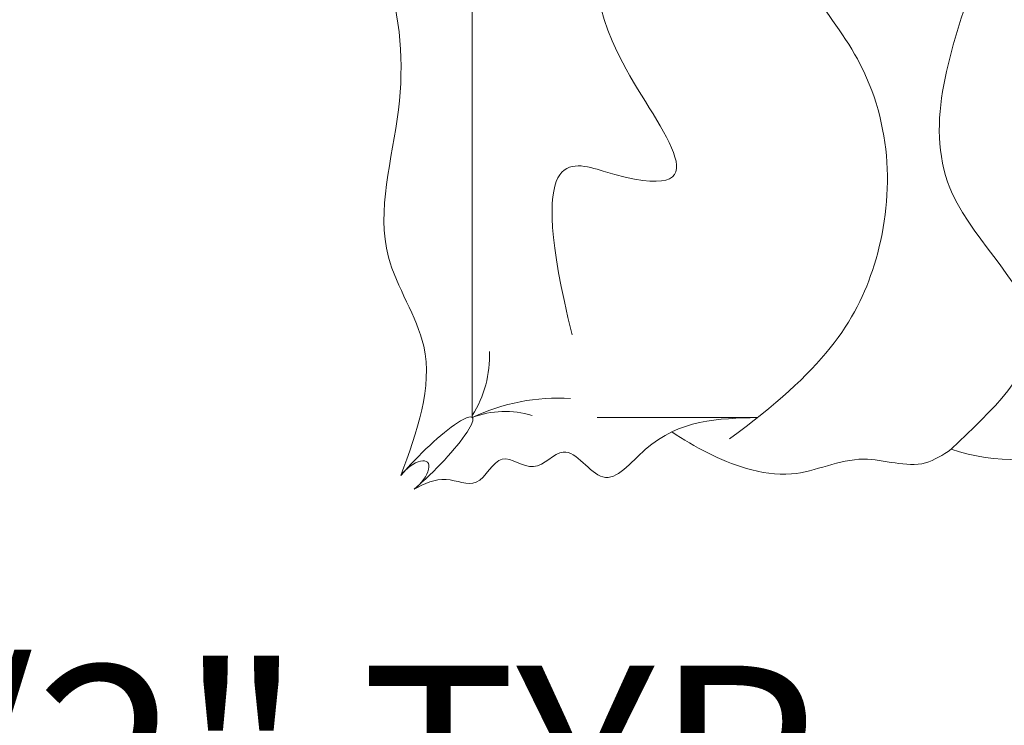
# Model space of a CAD drawing. Units: inches. Extents: x 2083 to 3317, y 1141 to 2115.
# Tile 120 of 256: x 3006 to 3068, y 1283 to 1327. Entities that reach past the tile are written whole.
import ezdxf

# ---------------------------------------------------------------- set-up
doc = ezdxf.new("R2010")
doc.units = ezdxf.units.IN
for name, color, linetype, lineweight in [('A-ANNO-DIMS', 2, 'Continuous', 18), ('A-FURN', 8, 'Continuous', 18), ('www.cadblocksfree.com', 7, 'Continuous', 9)]:
    doc.layers.add(name, color=color, linetype=linetype, lineweight=lineweight)
doc.layers.add('A-WALL-PATT', color=251, linetype='Continuous', lineweight=13, true_color=0x636466)
doc.styles.get("Standard").update_dxf_attribs({"font": 'arial.ttf'})
doc.dimstyles.new('ISO-25', dxfattribs={"dimtxt": 12, "dimasz": 12, "dimexe": 1.25, "dimexo": 0.625, "dimtad": 1, "dimlunit": 3, "dimtxsty": 'Standard', "dimcen": 2.5, "dimadec": 0, "dimazin": 0, "dimtfac": 1, "dimtmove": 0, "dimatfit": 3, "dimfxl": 1, "dimarcsym": 0})

# ---------------------------------------------------------------- blocks, each defined once
blk = doc.blocks.new('bed')
at = {"layer": 'www.cadblocksfree.com', "ltscale": 0.2}
for p, q in [((3426.379, 1399.908), (3426.379, 1410.814)), ((3363.387, 1391.414), (3426.379, 1391.414))]:
    blk.add_line(p, q, dxfattribs=at)
for centre, radius, start, end in [((3416.575, 1428.082), 12.646, 341.02679, 23.77822), ((3438.819, 1397.314), 13.768, 176.75247, 205.37301), ((3432.135, 1393.639), 6.173, 162.64747, 201.1361), ((3422.111, 1384.801), 7.798, 58.00129, 91.65506)]:
    blk.add_arc(centre, radius, start, end, dxfattribs=at)
for centre, major_axis, ratio, start_param, end_param in [((3429.422, 1388.371), (-3.043, 3.043), 0.168252, 4.250342, 8.316029), ((3430.477, 1387.316), (-1.055, 1.055), 0.453532, 4.422107, 8.144264)]:
    blk.add_ellipse(centre, major_axis=major_axis, ratio=ratio, start_param=start_param, end_param=end_param, dxfattribs=at)
for points, knots in [([(3365.512, 1424.213), (3370.519, 1427.004), (3381.149, 1429.825), (3396.214, 1425.866), (3410.541, 1420.654), (3420.273, 1432.695), (3425.882, 1426.771), (3428.534, 1423.97)], [0.099185, 0.099185, 0.099185, 0.099185, 0.523647, 0.927087, 1.289918, 1.564439, 1.810555, 1.810555, 1.810555, 1.810555]), ([(3428.534, 1423.97), (3428.914, 1423.397), (3430.098, 1421.613), (3428.491, 1417.656), (3430.593, 1413.794), (3429.801, 1409.122), (3428.396, 1406.564), (3427.355, 1404.971)], [0, 0, 0, 0, 0.050513, 0.157399, 0.2842023, 0.3628173, 0.5066917, 0.5066917, 0.5066917, 0.5066917]), ([(3362.057, 1409.866), (3363.638, 1413.65), (3372.978, 1421.337), (3389.682, 1406.045), (3402.396, 1419.984), (3416.037, 1420.167), (3423.233, 1415.231), (3427.827, 1408.899)], [0.029901, 0.029901, 0.029901, 0.029901, 0.276967, 0.797115, 1.093669, 1.464666, 1.788489, 1.788489, 1.788489, 1.788489]), ([(3431.237, 1387.473), (3430.882, 1388.172), (3430.205, 1389.505), (3431.478, 1391.985), (3428.294, 1393.194), (3430.501, 1395.689), (3427.558, 1397.866), (3431.841, 1400.386), (3426.535, 1404.33), (3426.443, 1408.152), (3426.379, 1410.814)], [0, 0, 0, 0, 2.267059, 4.324559, 6.685584, 8.878641, 11.121502, 14.300359, 17.755284, 25.682856, 25.682856, 25.682856, 25.682856]), ([(3368.632, 1397.839), (3375.978, 1400.489), (3385.349, 1402.757), (3397.531, 1395.273), (3413.593, 1410.377), (3407.806, 1395.019), (3420.759, 1398.2)], [0.029901, 0.029901, 0.029901, 0.029901, 0.276967, 0.797115, 1.093669, 1.16836, 1.16836, 1.16836, 1.16836]), ([(3430.32, 1386.556), (3427.327, 1387.653), (3422.148, 1389.55), (3414.529, 1384.137), (3405.607, 1387.046), (3396.29, 1386.314), (3386.838, 1381.282), (3377.742, 1390.272), (3370.778, 1384.799), (3364.626, 1383.966), (3363.275, 1388.265), (3360.778, 1387.151), (3359.446, 1386.556)], [0, 0, 0, 0, 8.93042, 15.449194, 25.485629, 34.878505, 43.598887, 54.554403, 64.16647, 67.461673, 70.610457, 74.213583, 74.213583, 74.213583, 74.213583])]:
    blk.add_open_spline(points, degree=3, knots=knots, dxfattribs=at)
blk = doc.blocks.new('*D26')
at = {"layer": 'A-ANNO-DIMS', "color": 0, "lineweight": -2, "transparency": 16777216}
for p, q in [((3088.986, 1274.915), (3088.986, 1270.952)), ((3111.24, 1274.915), (3111.24, 1270.952)), ((3076.986, 1272.202), (2840.262, 1272.202)), ((3111.24, 1272.202), (3088.986, 1272.202)), ((3123.24, 1272.202), (3135.24, 1272.202))]:
    blk.add_line(p, q, dxfattribs=at)
at = {"layer": 'A-ANNO-DIMS', "color": 0, "transparency": 16777216}
for points in [[(3076.986, 1274.202), (3076.986, 1270.202), (3088.986, 1272.202)], [(3123.24, 1274.202), (3123.24, 1270.202), (3111.24, 1272.202)]]:
    blk.add_solid(points, dxfattribs=at)
at = {"layer": 'Defpoints', "color": 0, "transparency": 16777216}
for p in [(3088.986, 1275.54), (3111.24, 1275.54), (3088.986, 1272.202)]:
    blk.add_point(p, dxfattribs=at)
at = {"layer": 'A-ANNO-DIMS', "color": 0, "transparency": 16777216, "insert": (2952.624, 1279.032), "char_height": 12, "attachment_point": 5}
blk.add_mtext('NIGHTSTAND 1\'-10 1/2" TYP.', dxfattribs=at)

msp = doc.modelspace()

# ---------------------------------------------------------------- hatches: boundary and pattern name
at = {"layer": 'A-WALL-PATT'}
h = msp.add_hatch(color=256, dxfattribs=at)
h.dxf.hatch_style = 1
h.paths.add_polyline_path([(3126.96, 2020.761), (2748.96, 2020.761), (2604.96, 2020.761), (2226.96, 2020.761), (2226.96, 1702.761), (2466.96, 1702.761), (2466.96, 1582.761), (2418.96, 1582.761), (2418.96, 1477.761), (2226.96, 1477.761), (2226.96, 1263.261), (2544.96, 1263.261), (2544.96, 1411.761), (2604.96, 1411.761), (2685.96, 1411.761), (2685.96, 1420.761), (2604.96, 1420.761), (2604.96, 1573.761), (2604.96, 1702.761), (2604.96, 2011.761), (2748.96, 2011.761), (2748.96, 1702.761), (2862.96, 1702.761), (2862.96, 1621.761), (2871.96, 1621.761), (2871.96, 1702.761), (2883.96, 1702.761), (2883.96, 1706.939, -0.026459), (2883.96, 1711.761), (2757.96, 1711.761), (2757.96, 1807.761), (2787.96, 1807.761), (2787.96, 1812.261), (2757.96, 1812.261), (2757.96, 2011.761), (2877.96, 2011.761), (2877.96, 1812.261), (2847.96, 1812.261), (2847.96, 1807.761), (2889.836, 1807.761), (2889.836, 1812.261), (2882.46, 1812.261), (2882.46, 2011.761), (3117.96, 2011.761), (3117.96, 1812.261), (2937.836, 1812.261), (2937.836, 1807.761), (2995.71, 1807.761), (2995.71, 1796.118), (3000.21, 1796.118), (3000.21, 1807.761), (3117.96, 1807.761), (3117.96, 1711.761), (3000.21, 1711.761), (3000.21, 1760.118), (2998.573, 1760.118, -0.020711), (2995.71, 1760.118), (2995.71, 1711.761), (2931.96, 1711.761), (2931.96, 1702.761), (3126.96, 1702.761)])
h.paths.add_polyline_path([(2471.46, 2011.761), (2471.46, 1810.011), (2462.717, 1810.011), (2462.717, 1805.511), (2505.96, 1805.511), (2505.96, 1810.011), (2475.96, 1810.011), (2475.96, 2011.761), (2595.96, 2011.761), (2595.96, 1810.011), (2565.96, 1810.011), (2565.96, 1805.511), (2595.96, 1805.511), (2595.96, 1711.761), (2235.96, 1711.761), (2235.96, 1805.511), (2353.71, 1805.511), (2353.71, 1796.054), (2358.21, 1796.054), (2358.21, 1805.511), (2414.717, 1805.511), (2414.717, 1810.011), (2235.96, 1810.011), (2235.96, 2011.761)], flags=16)
h.paths.add_polyline_path([(2270.205, 1994.61), (2270.205, 1970.61), (2246.205, 1970.61), (2246.205, 1994.61)], flags=0)
edge = h.paths.add_edge_path(flags=0)
edge.add_ellipse((2332.027, 1899.798), major_axis=(-3.043, 3.043), ratio=0.168252, start_angle=-161.33217, end_angle=-156.30711, ccw=False)
edge.add_ellipse((2333.082, 1898.744), major_axis=(-1.055, 1.055), ratio=0.453532, start_angle=-123.37102, end_angle=-94.15911)
edge = h.paths.add_edge_path(flags=0)
edge.add_ellipse((2332.027, 1968.876), major_axis=(3.043, 3.043), ratio=0.168252, start_angle=18.66783, end_angle=23.69289)
edge.add_spline(control_points=[(2332.926, 1970.691), (2332.227, 1970.336), (2330.894, 1969.659), (2328.413, 1970.932), (2327.204, 1967.749), (2324.71, 1969.956), (2322.533, 1967.012), (2320.013, 1971.296), (2317.68, 1968.158), (2316.041, 1967.102), (2315.427, 1966.81)], knot_values=[0, 0, 0, 0, 2.267059, 4.324559, 6.685584, 8.878641, 11.121502, 14.300359, 17.755284, 19.732645, 19.732645, 19.732645, 19.732645], degree=3, periodic=0)
edge.add_ellipse((2332.027, 1968.876), major_axis=(3.043, 3.043), ratio=0.168252, start_angle=18.66783, end_angle=23.69289, ccw=False)
edge.add_ellipse((2333.082, 1969.931), major_axis=(1.055, 1.055), ratio=0.453532, start_angle=56.62898, end_angle=85.84089, ccw=False)
edge = h.paths.add_edge_path(flags=0)
edge.add_spline(control_points=[(2296.428, 1967.988), (2293.628, 1965.336), (2287.704, 1959.727), (2299.744, 1949.996), (2294.533, 1935.669), (2290.573, 1920.604), (2293.394, 1909.974), (2296.185, 1904.967)], knot_values=[0.099185, 0.099185, 0.099185, 0.099185, 0.345301, 0.619822, 0.982653, 1.386093, 1.810555, 1.810555, 1.810555, 1.810555], degree=3, periodic=0)
edge.add_spline(control_points=[(2296.185, 1904.967), (2297.384, 1902.619), (2298.001, 1901.949), (2298.553, 1901.468)], knot_values=[0.006246, 0.006246, 0.006246, 0.006246, 0.055476, 0.055476, 0.055476, 0.055476], degree=3, periodic=0)
edge.add_spline(control_points=[(2298.553, 1901.468), (2297.259, 1900.923), (2295.225, 1900.232), (2293.06, 1900.614), (2292.101, 1900.788), (2292.09, 1900.791)], knot_values=[0.312835, 0.312835, 0.312835, 0.312835, 0.40178, 0.474987, 0.475903, 0.475903, 0.475903, 0.475903], degree=3, periodic=0)
edge.add_arc((2292.794, 1904.664), 3.937, 215.4209, 259.69818, ccw=False)
edge.add_spline(control_points=[(2289.585, 1902.382), (2289.477, 1902.535), (2289.368, 1902.688), (2289.261, 1902.841)], knot_values=[0.102872, 0.102872, 0.102872, 0.102872, 0.116896, 0.116896, 0.116896, 0.116896], degree=3, periodic=0)
edge.add_spline(control_points=[(2289.261, 1902.841), (2288.687, 1902.55), (2287.64, 1902.02), (2285.881, 1901.874), (2283.853, 1901.504), (2281.72, 1899.711), (2278.467, 1899.493), (2276.157, 1901.883), (2272.259, 1899.804), (2267.778, 1901.843), (2262.244, 1900.184), (2257.415, 1901.782), (2254.318, 1900.726), (2253.178, 1900.337)], knot_values=[0, 0, 0, 0, 1.907977, 3.477176, 5.261074, 7.972851, 11.680248, 13.717921, 16.939592, 22.789562, 27.502503, 33.595215, 37.145618, 37.145618, 37.145618, 37.145618], degree=3, periodic=0)
edge.add_line((2253.178, 1900.337), (2250.244, 1902.841))
edge.add_line((2250.244, 1902.841), (2250.244, 1965.833))
edge.add_line((2250.244, 1965.833), (2253.178, 1968.337))
edge.add_spline(control_points=[(2253.178, 1968.337), (2254.318, 1967.948), (2257.415, 1966.892), (2262.244, 1968.49), (2267.778, 1966.831), (2271.527, 1968.537), (2273.876, 1967.828), (2274.207, 1967.728)], knot_values=[0, 0, 0, 0, 0.09018, 0.244935, 0.364644, 0.513233, 0.537855, 0.537855, 0.537855, 0.537855], degree=3, periodic=0)
edge.add_arc((2274.353, 1963.793), 3.937, 72.05113, 92.12795, ccw=False)
edge.add_arc((2281.297, 1985.23), 18.596, 252.05113, 288.56572)
edge.add_arc((2292.317, 1956.029), 12.646, 71.02679, 113.77822, ccw=False)
edge = h.paths.add_edge_path(flags=0)
edge.add_spline(control_points=[(2274.899, 1951.856), (2275.066, 1951.617), (2275.233, 1951.377), (2275.398, 1951.136)], knot_values=[1.409916, 1.409916, 1.409916, 1.409916, 1.43159, 1.43159, 1.43159, 1.43159], degree=3, periodic=0)
edge.add_spline(control_points=[(2275.398, 1951.136), (2275.792, 1950.562), (2276.179, 1949.984), (2276.546, 1949.397)], knot_values=[1.358238, 1.358238, 1.358238, 1.358238, 1.409916, 1.409916, 1.409916, 1.409916], degree=3, periodic=0)
edge.add_line((2276.546, 1949.397), (2277.437, 1947.862))
edge.add_spline(control_points=[(2277.437, 1947.862), (2276.304, 1945.673), (2274.64, 1942.427), (2274.632, 1938.094), (2272.799, 1930.852), (2274.356, 1943.897), (2275.948, 1947.923), (2276.546, 1949.397)], knot_values=[0.005632, 0.005632, 0.005632, 0.005632, 0.186014, 0.266002, 0.357087, 0.59639, 0.739732, 0.739732, 0.739732, 0.739732], degree=3, periodic=0)
edge.add_spline(control_points=[(2276.546, 1949.397), (2276.179, 1949.984), (2275.792, 1950.562), (2275.398, 1951.136)], knot_values=[1.358238, 1.358238, 1.358238, 1.358238, 1.409916, 1.409916, 1.409916, 1.409916], degree=3, periodic=0)
edge.add_spline(control_points=[(2275.398, 1951.136), (2274.943, 1950.08), (2274.208, 1948.025), (2273.935, 1944.851), (2272.469, 1937.627), (2273.466, 1945.696), (2274.701, 1951.059), (2274.899, 1951.856)], knot_values=[0.104364, 0.104364, 0.104364, 0.104364, 0.189636, 0.269624, 0.36071, 0.600013, 0.644622, 0.644622, 0.644622, 0.644622], degree=3, periodic=0)
h.paths.add_polyline_path([(2269.168, 1963.128, -0.357527), (2268.171, 1960.976, -0.092561), (2268.171, 1939.436, -0.357527), (2269.168, 1937.285, -0.357527), (2267.016, 1938.282, -0.164785), (2254.686, 1938.282, -0.357527), (2252.534, 1937.285, -0.357527), (2253.531, 1939.436, -0.092561), (2253.531, 1960.976, -0.357527), (2252.534, 1963.128, -0.357527), (2254.686, 1962.131, -0.164785), (2267.016, 1962.131, -0.357527)], flags=0)
h.paths.add_polyline_path([(2248.874, 1967.802), (2248.874, 1957.028), (2249.458, 1957.028), (2249.458, 1911.647), (2248.874, 1911.647), (2248.874, 1900.873), (2246.512, 1900.873, 0.197327), (2244.15, 1902.457), (2244.15, 1966.218, 0.197327), (2246.512, 1967.802)], flags=0)
h.paths.add_polyline_path([(2269.168, 1931.389, -0.357527), (2268.171, 1929.238, -0.092561), (2268.171, 1907.698, -0.357527), (2269.168, 1905.547, -0.357527), (2267.016, 1906.544, -0.164785), (2254.686, 1906.544, -0.357527), (2252.534, 1905.547, -0.357527), (2253.531, 1907.698, -0.092561), (2253.531, 1929.238, -0.357527), (2252.534, 1931.389, -0.357527), (2254.686, 1930.392, -0.164785), (2267.016, 1930.392, -0.357527)], flags=0)
edge = h.paths.add_edge_path(flags=0)
edge.add_spline(control_points=[(2276.197, 1906.724), (2276.168, 1909.029), (2276.114, 1913.372), (2270.598, 1924.925), (2273.905, 1919.013), (2275.922, 1916.262), (2275.475, 1912.402), (2277.258, 1910.381), (2276.696, 1908.225), (2276.646, 1906.813), (2276.618, 1906.008)], knot_values=[0, 0, 0, 0, 8.61026, 16.221274, 18.843057, 23.804898, 27.440828, 29.356102, 31.203478, 33.650687, 33.650687, 33.650687, 33.650687], degree=3, periodic=0)
edge.add_spline(control_points=[(2276.618, 1906.008), (2276.623, 1905.624), (2276.498, 1904.629), (2275.442, 1903.855), (2274.937, 1903.08), (2274.859, 1902.841)], knot_values=[0.156488, 0.156488, 0.156488, 0.156488, 0.184398, 0.231376, 0.250598, 0.250598, 0.250598, 0.250598], degree=3, periodic=0)
edge.add_line((2274.859, 1902.841), (2276.506, 1902.841))
edge.add_spline(control_points=[(2276.506, 1902.841), (2276.788, 1903.085), (2277.665, 1904.125), (2278.25, 1904.341), (2277.654, 1908.527), (2278.156, 1906.228), (2278.1, 1905.286), (2278.847, 1904.069), (2277.857, 1903.415), (2277.874, 1902.991), (2277.904, 1902.841)], knot_values=[0.059574, 0.059574, 0.059574, 0.059574, 0.080753, 0.103741, 0.16972, 0.176036, 0.207137, 0.240474, 0.262341, 0.27366, 0.27366, 0.27366, 0.27366], degree=3, periodic=0)
edge.add_line((2277.904, 1902.841), (2280.03, 1902.841))
edge.add_spline(control_points=[(2280.03, 1902.841), (2279.888, 1903.088), (2279.499, 1903.982), (2280.152, 1905.939), (2278.104, 1909.658), (2279.762, 1907.185), (2280.328, 1904.875), (2280.485, 1903.49), (2281.463, 1903.249), (2281.758, 1902.936), (2281.834, 1902.841)], knot_values=[0.013856, 0.013856, 0.013856, 0.013856, 0.034874, 0.088867, 0.107879, 0.126738, 0.158714, 0.193757, 0.217487, 0.226722, 0.226722, 0.226722, 0.226722], degree=3, periodic=0)
edge.add_spline(control_points=[(2281.834, 1902.841), (2281.788, 1902.827), (2281.647, 1902.783), (2281.396, 1902.859), (2281.088, 1902.985), (2280.721, 1903.061), (2280.333, 1903.026), (2280.125, 1902.899), (2280.03, 1902.841)], knot_values=[0, 0, 0, 0, 0.14413, 0.435517, 0.749276, 1.153046, 1.548371, 1.878348, 1.878348, 1.878348, 1.878348], degree=3, periodic=0)
edge.add_line((2280.03, 1902.841), (2277.904, 1902.841))
edge.add_spline(control_points=[(2277.904, 1902.841), (2277.893, 1902.796), (2277.865, 1902.68), (2277.607, 1902.687), (2277.274, 1902.801), (2276.838, 1902.62), (2276.584, 1902.789), (2276.506, 1902.841)], knot_values=[0, 0, 0, 0, 0.127189, 0.326199, 0.628009, 1.24357, 1.515331, 1.515331, 1.515331, 1.515331], degree=3, periodic=0)
edge.add_line((2276.506, 1902.841), (2274.859, 1902.841))
edge.add_spline(control_points=[(2274.859, 1902.841), (2274.814, 1902.899), (2274.725, 1903.013), (2274.493, 1903.119), (2274.244, 1902.961), (2273.937, 1903.185), (2273.614, 1902.983), (2273.408, 1902.883), (2273.322, 1902.841)], knot_values=[0, 0, 0, 0, 0.21843, 0.436957, 0.687977, 0.990379, 1.398396, 1.69185, 1.69185, 1.69185, 1.69185], degree=3, periodic=0)
edge.add_spline(control_points=[(2273.322, 1902.841), (2273.617, 1903.446), (2274.274, 1904.538), (2276.027, 1904.574), (2276.207, 1906.584), (2276.197, 1906.724)], knot_values=[0.012227, 0.012227, 0.012227, 0.012227, 0.059472, 0.106218, 0.134458, 0.134458, 0.134458, 0.134458], degree=3, periodic=0)
h.paths.add_polyline_path([(2270.776, 1897.79), (2270.776, 1873.79), (2246.776, 1873.79), (2246.776, 1897.79)], flags=0)
h.paths.add_polyline_path([(2353.71, 1760.005), (2353.71, 1760.054), (2358.21, 1760.054, -0.033729)], flags=0)
h.paths.add_polyline_path([(2321.819, 1737.529), (2341.995, 1737.529, -0.414214), (2343.203, 1736.321), (2343.203, 1721.021, -0.414214), (2341.995, 1719.813), (2321.819, 1719.813, -0.414214), (2320.611, 1721.021), (2320.611, 1736.321, -0.414214)], flags=0)
h.paths.add_polyline_path([(2324.235, 1736.321), (2339.579, 1736.321, -0.414214), (2341.995, 1733.905), (2341.995, 1725.45, -0.414214), (2339.579, 1723.034), (2333.681, 1723.034), (2333.845, 1722.045, -0.870646), (2335.425, 1721.826, -0.767327), (2333.923, 1721.423), (2331.291, 1721.423, -0.767327), (2329.788, 1721.826, -0.870646), (2331.368, 1722.045), (2331.533, 1723.034), (2324.235, 1723.034, -0.414214), (2321.819, 1725.45), (2321.819, 1733.905, -0.414214)], flags=0)
h.paths.add_polyline_path([(2570.484, 1928.615), (2589.684, 1928.615), (2590.169, 1928.615), (2590.169, 1904.993), (2570.484, 1904.993)], flags=0)
h.paths.add_polyline_path([(2574.447, 1927.264, -1), (2572.829, 1927.264, -1)], flags=0)
h.paths.add_polyline_path([(2573.09, 1926.941), (2573.925, 1927.776), (2574.148, 1927.553), (2573.313, 1926.718)], flags=0)
h.paths.add_polyline_path([(2578.779, 1919.73, -1), (2571.592, 1919.73, -1)], flags=0)
h.paths.add_polyline_path([(2578.385, 1919.73, -1), (2571.985, 1919.73, -1)], flags=0)
h.paths.add_polyline_path([(2331.596, 1729.476, -1), (2333.618, 1729.476, -1)], flags=0)
h.paths.add_polyline_path([(2578.034, 1927.264, -1), (2576.416, 1927.264, -1)], flags=0)
h.paths.add_polyline_path([(2576.689, 1927.531), (2576.912, 1927.754), (2577.747, 1926.919), (2577.524, 1926.696)], flags=0)
h.paths.add_polyline_path([(2578.139, 1909.86, -1), (2572.232, 1909.86, -1)], flags=0)
h.paths.add_polyline_path([(2577.745, 1909.86, -1), (2572.625, 1909.86, -1)], flags=0)
h.paths.add_polyline_path([(2583.798, 1927.264, -1), (2582.179, 1927.264, -1)], flags=0)
h.paths.add_polyline_path([(2582.719, 1927.754), (2583.554, 1926.919), (2583.331, 1926.696), (2582.496, 1927.531)], flags=0)
h.paths.add_polyline_path([(2582.496, 1927.531), (2582.719, 1927.754), (2583.554, 1926.919), (2583.331, 1926.696)], flags=0)
h.paths.add_polyline_path([(2587.739, 1920.53, -1), (2581.832, 1920.53, -1)], flags=0)
h.paths.add_polyline_path([(2587.345, 1920.53, -1), (2582.225, 1920.53, -1)], flags=0)
h.paths.add_polyline_path([(2587.385, 1927.264, -1), (2585.766, 1927.264, -1)], flags=0)
h.paths.add_polyline_path([(2586.082, 1926.98), (2586.917, 1927.815), (2587.14, 1927.593), (2586.305, 1926.758)], flags=0)
h.paths.add_polyline_path([(2588.379, 1910.66, -1), (2581.192, 1910.66, -1)], flags=0)
h.paths.add_polyline_path([(2587.985, 1910.66, -1), (2581.585, 1910.66, -1)], flags=0)
h.paths.add_polyline_path([(2417.168, 1729.478), (2437.344, 1729.478, -0.414214), (2438.552, 1728.27), (2438.552, 1712.969, -0.414214), (2437.344, 1711.761), (2417.168, 1711.761, -0.414214), (2415.96, 1712.969), (2415.96, 1728.27, -0.414214)], flags=0)
h.paths.add_polyline_path([(2419.584, 1728.27), (2434.928, 1728.27, -0.414214), (2437.344, 1725.854), (2437.344, 1717.398, -0.414214), (2434.928, 1714.983), (2429.029, 1714.983), (2429.194, 1713.994, -0.870646), (2430.774, 1713.775, -0.767327), (2429.271, 1713.372), (2426.64, 1713.372, -0.767327), (2425.137, 1713.775, -0.870646), (2426.717, 1713.994), (2426.882, 1714.983), (2419.584, 1714.983, -0.414214), (2417.168, 1717.398), (2417.168, 1725.854, -0.414214)], flags=0)
h.paths.add_polyline_path([(2419.584, 1728.27), (2434.928, 1728.27, -0.414214), (2437.344, 1725.854), (2437.344, 1717.398, -0.414214), (2434.928, 1714.983), (2429.029, 1714.983), (2428.358, 1719.009), (2427.553, 1719.009), (2426.882, 1714.983), (2419.584, 1714.983, -0.414214), (2417.168, 1717.398), (2417.168, 1725.854, -0.414214)], flags=0)
h.paths.add_polyline_path([(2426.944, 1721.425, -1), (2428.967, 1721.425, -1)], flags=0)
h.paths.add_polyline_path([(2475.96, 1702.761), (2595.96, 1702.761), (2595.96, 1582.761), (2475.96, 1582.761)], flags=16)
h.paths.add_polyline_path([(2427.96, 1573.761), (2595.96, 1573.761), (2595.96, 1468.761), (2595.96, 1420.761), (2384.46, 1420.761), (2384.46, 1468.761), (2427.96, 1468.761)], flags=16)
h.paths.add_polyline_path([(2379.96, 1468.761), (2379.96, 1420.761), (2235.96, 1420.761), (2235.96, 1468.761)], flags=16)
h.paths.add_polyline_path([(2317.816, 1466.696), (2337.992, 1466.696, -0.414214), (2339.2, 1465.488), (2339.2, 1450.187, -0.414214), (2337.992, 1448.979), (2317.816, 1448.979, -0.414214), (2316.608, 1450.187), (2316.608, 1465.488, -0.414214)], flags=0)
h.paths.add_polyline_path([(2320.232, 1465.488), (2335.576, 1465.488, -0.414214), (2337.992, 1463.072), (2337.992, 1454.616, -0.414214), (2335.576, 1452.2), (2329.677, 1452.2), (2329.842, 1451.212, -0.870646), (2331.422, 1450.992, -0.767327), (2329.92, 1450.59), (2327.288, 1450.59, -0.767327), (2325.785, 1450.992, -0.870646), (2327.365, 1451.212), (2327.53, 1452.2), (2320.232, 1452.2, -0.414214), (2317.816, 1454.616), (2317.816, 1463.072, -0.414214)], flags=0)
h.paths.add_polyline_path([(2320.232, 1465.488), (2335.576, 1465.488, -0.414214), (2337.992, 1463.072), (2337.992, 1454.616, -0.414214), (2335.576, 1452.2), (2329.677, 1452.2), (2329.006, 1456.227), (2328.201, 1456.227), (2327.53, 1452.2), (2320.232, 1452.2, -0.414214), (2317.816, 1454.616), (2317.816, 1463.072, -0.414214)], flags=0)
h.paths.add_polyline_path([(2327.593, 1458.643, -1), (2329.615, 1458.643, -1)], flags=0)
h.paths.add_polyline_path([(2244.412, 1433.34), (2241.921, 1433.34, -0.414214), (2240.018, 1435.244), (2240.018, 1440.953, -0.414211), (2241.921, 1442.856), (2244.412, 1442.856, -1.976472)], flags=0)
h.paths.add_polyline_path([(2245.357, 1434.398, -0.414214), (2245.357, 1441.799, -2.144098)], flags=0)
h.paths.add_polyline_path([(2535.96, 1416.261), (2535.96, 1272.261), (2235.96, 1272.261), (2235.96, 1416.261)], flags=16)
h.paths.add_polyline_path([(2260.12, 1384.293), (2260.12, 1362.039), (2237.865, 1362.039), (2237.865, 1384.293)], flags=0)
edge = h.paths.add_edge_path(flags=0)
edge.add_line((2318.252, 1362.093), (2318.146, 1362.001))
edge.add_ellipse((2317.445, 1360.431), major_axis=(2.822, 2.822), ratio=0.168252, start_angle=18.66783, end_angle=20.94813, ccw=False)
edge.add_ellipse((2318.423, 1361.409), major_axis=(0.978, 0.978), ratio=0.453532, start_angle=56.62898, end_angle=70.2262, ccw=False)
edge = h.paths.add_edge_path(flags=0)
edge.add_line((2319.107, 1295.571), (2319.015, 1295.677))
edge.add_ellipse((2317.445, 1296.378), major_axis=(-2.822, 2.822), ratio=0.168252, start_angle=-161.33217, end_angle=-159.05187, ccw=False)
edge.add_ellipse((2318.423, 1295.4), major_axis=(-0.978, 0.978), ratio=0.453532, start_angle=-123.37102, end_angle=-109.7738)
edge = h.paths.add_edge_path(flags=0)
edge.add_spline(control_points=[(2284.21, 1301.17), (2284.581, 1300.445), (2284.891, 1299.892), (2285.16, 1299.461)], knot_values=[0.039066, 0.039066, 0.039066, 0.039066, 0.055476, 0.055476, 0.055476, 0.055476], degree=3, periodic=0)
edge.add_line((2285.16, 1299.461), (2284.21, 1301.17))
edge = h.paths.add_edge_path(flags=0)
edge.add_line((2280.412, 1297.298), (2283.37, 1297.036))
edge.add_line((2283.37, 1297.036), (2286.406, 1297.926))
edge.add_spline(control_points=[(2286.406, 1297.926), (2285.305, 1297.463), (2284.345, 1297.129), (2283.37, 1297.036)], knot_values=[0.394369, 0.394369, 0.394369, 0.394369, 0.475903, 0.475903, 0.475903, 0.475903], degree=3, periodic=0)
edge.add_spline(control_points=[(2283.37, 1297.036), (2283.281, 1297.028), (2282.316, 1296.957), (2281.313, 1297.134), (2280.423, 1297.296), (2280.412, 1297.298)], knot_values=[0.312835, 0.312835, 0.312835, 0.312835, 0.320246, 0.393453, 0.394369, 0.394369, 0.394369, 0.394369], degree=3, periodic=0)
edge = h.paths.add_edge_path(flags=0)
edge.add_line((2284.436, 1359.607), (2280.446, 1355.328))
edge.add_line((2280.446, 1355.328), (2279.58, 1351.018))
edge.add_line((2279.58, 1351.018), (2282.413, 1346.58))
edge.add_spline(control_points=[(2282.413, 1346.58), (2283.153, 1345.589), (2284.253, 1344.029), (2284.801, 1342.387), (2284.935, 1341.806)], knot_values=[1.240098, 1.240098, 1.240098, 1.240098, 1.332892, 1.382712, 1.382712, 1.382712, 1.382712], degree=3, periodic=0)
edge.add_spline(control_points=[(2284.935, 1341.806), (2285.319, 1340.141), (2285.233, 1338.409), (2284.91, 1336.654)], knot_values=[1.097484, 1.097484, 1.097484, 1.097484, 1.240098, 1.240098, 1.240098, 1.240098], degree=3, periodic=0)
edge.add_spline(control_points=[(2284.91, 1336.654), (2284.587, 1334.899), (2284.027, 1333.12), (2283.463, 1331.361)], knot_values=[0.95487, 0.95487, 0.95487, 0.95487, 1.097484, 1.097484, 1.097484, 1.097484], degree=3, periodic=0)
edge.add_line((2283.463, 1331.361), (2281.89, 1326.153))
edge.add_line((2281.89, 1326.153), (2280.756, 1321.056))
edge.add_line((2280.756, 1321.056), (2280.299, 1316.002))
edge.add_line((2280.299, 1316.002), (2280.716, 1310.95))
edge.add_line((2280.716, 1310.95), (2282.028, 1305.972))
edge.add_line((2282.028, 1305.972), (2284.21, 1301.17))
edge.add_spline(control_points=[(2284.21, 1301.17), (2283.341, 1302.73), (2282.612, 1304.336), (2282.028, 1305.972)], knot_values=[0.099185, 0.099185, 0.099185, 0.099185, 0.241799, 0.241799, 0.241799, 0.241799], degree=3, periodic=0)
edge.add_spline(control_points=[(2282.028, 1305.972), (2281.444, 1307.608), (2281.005, 1309.273), (2280.716, 1310.95)], knot_values=[0.241799, 0.241799, 0.241799, 0.241799, 0.384413, 0.384413, 0.384413, 0.384413], degree=3, periodic=0)
edge.add_spline(control_points=[(2280.716, 1310.95), (2280.433, 1312.588), (2280.289, 1314.277), (2280.299, 1315.962), (2280.299, 1316.002)], knot_values=[0.384413, 0.384413, 0.384413, 0.384413, 0.523647, 0.527028, 0.527028, 0.527028, 0.527028], degree=3, periodic=0)
edge.add_spline(control_points=[(2280.299, 1316.002), (2280.312, 1317.687), (2280.478, 1319.368), (2280.756, 1321.056)], knot_values=[0.527028, 0.527028, 0.527028, 0.527028, 0.669642, 0.669642, 0.669642, 0.669642], degree=3, periodic=0)
edge.add_spline(control_points=[(2280.756, 1321.056), (2281.035, 1322.744), (2281.426, 1324.44), (2281.89, 1326.153)], knot_values=[0.669642, 0.669642, 0.669642, 0.669642, 0.812256, 0.812256, 0.812256, 0.812256], degree=3, periodic=0)
edge.add_spline(control_points=[(2281.89, 1326.153), (2282.264, 1327.533), (2282.788, 1329.262), (2283.353, 1331.018), (2283.463, 1331.361)], knot_values=[0.812256, 0.812256, 0.812256, 0.812256, 0.927087, 0.95487, 0.95487, 0.95487, 0.95487], degree=3, periodic=0)
edge.add_line((2283.463, 1331.361), (2284.91, 1336.654))
edge.add_line((2284.91, 1336.654), (2284.935, 1341.806))
edge.add_line((2284.935, 1341.806), (2282.413, 1346.58))
edge.add_spline(control_points=[(2282.413, 1346.58), (2281.275, 1348.104), (2280.078, 1349.57), (2279.58, 1351.018)], knot_values=[1.382712, 1.382712, 1.382712, 1.382712, 1.525326, 1.525326, 1.525326, 1.525326], degree=3, periodic=0)
edge.add_spline(control_points=[(2279.58, 1351.018), (2279.443, 1351.415), (2279.136, 1352.857), (2279.735, 1354.29), (2280.446, 1355.328)], knot_values=[1.525326, 1.525326, 1.525326, 1.525326, 1.564439, 1.667941, 1.667941, 1.667941, 1.667941], degree=3, periodic=0)
edge.add_spline(control_points=[(2280.446, 1355.328), (2281.426, 1356.758), (2282.931, 1358.183), (2284.436, 1359.607)], knot_values=[1.667941, 1.667941, 1.667941, 1.667941, 1.810555, 1.810555, 1.810555, 1.810555], degree=3, periodic=0)
edge.add_arc((2280.623, 1348.518), 11.726, 71.02679, 113.77822)
edge.add_arc((2270.405, 1375.595), 17.244, 252.05113, 288.56572, ccw=False)
edge.add_arc((2263.966, 1355.718), 3.651, 72.05113, 92.12795)
edge.add_arc((2263.966, 1355.718), 3.651, 92.12795, 177.98513)
edge.add_spline(control_points=[(2260.318, 1355.846), (2260.26, 1354.221), (2260.551, 1350.187), (2262.999, 1346.766), (2264.473, 1344.649)], knot_values=[1.43159, 1.43159, 1.43159, 1.43159, 1.564144, 1.770695, 1.770695, 1.770695, 1.770695], degree=3, periodic=0)
edge.add_line((2264.473, 1344.649), (2264.936, 1343.983))
edge.add_spline(control_points=[(2263.801, 1340.248), (2263.843, 1340.514), (2264.067, 1341.756), (2264.513, 1343.002), (2264.935, 1343.981)], knot_values=[0.53657, 0.53657, 0.53657, 0.53657, 0.559349, 0.644622, 0.644622, 0.644622, 0.644622], degree=3, periodic=0)
edge.add_spline(control_points=[(2264.935, 1343.981), (2265.118, 1343.715), (2265.299, 1343.448), (2265.477, 1343.179)], knot_values=[1.384077, 1.384077, 1.384077, 1.384077, 1.409916, 1.409916, 1.409916, 1.409916], degree=3, periodic=0)
edge.add_spline(control_points=[(2265.477, 1343.179), (2265.655, 1342.911), (2265.829, 1342.641), (2265.999, 1342.369)], knot_values=[1.358238, 1.358238, 1.358238, 1.358238, 1.384077, 1.384077, 1.384077, 1.384077], degree=3, periodic=0)
edge.add_line((2265.999, 1342.369), (2266.826, 1340.946))
edge.add_spline(control_points=[(2266.826, 1340.946), (2268.894, 1337.09), (2271.398, 1325.843), (2270.516, 1310.569), (2275.919, 1301.861), (2277.79, 1299.199)], knot_values=[0.116896, 0.116896, 0.116896, 0.116896, 0.472987, 1.050969, 1.313793, 1.313793, 1.313793, 1.313793], degree=3, periodic=0)
edge.add_spline(control_points=[(2277.79, 1299.199), (2277.839, 1299.128), (2277.889, 1299.057), (2277.94, 1298.987)], knot_values=[0.109884, 0.109884, 0.109884, 0.109884, 0.116896, 0.116896, 0.116896, 0.116896], degree=3, periodic=0)
edge.add_line((2277.94, 1298.987), (2277.789, 1299.199))
edge.add_spline(control_points=[(2277.789, 1299.199), (2277.257, 1298.929), (2276.286, 1298.438), (2275.039, 1298.334), (2274.383, 1298.239), (2274.215, 1298.209)], knot_values=[33.12187, 33.12187, 33.12187, 33.12187, 35.029056, 36.598255, 37.144827, 37.144827, 37.144827, 37.144827], degree=3, periodic=0)
edge.add_line((2274.215, 1298.209), (2273.073, 1297.893))
edge.add_spline(control_points=[(2273.073, 1297.893), (2272.323, 1297.58), (2271.039, 1296.511), (2269.248, 1296.226), (2268.423, 1296.375)], knot_values=[26.532584, 26.532584, 26.532584, 26.532584, 29.198919, 31.839101, 31.839101, 31.839101, 31.839101], degree=3, periodic=0)
edge.add_line((2268.423, 1296.375), (2263.879, 1297.458))
edge.add_spline(control_points=[(2263.879, 1297.458), (2263.556, 1297.359), (2261.86, 1296.839), (2260.239, 1297.282), (2258.933, 1297.516)], knot_values=[15.919551, 15.919551, 15.919551, 15.919551, 16.939592, 21.226067, 21.226067, 21.226067, 21.226067], degree=3, periodic=0)
edge.add_line((2258.933, 1297.516), (2254.055, 1297.329))
edge.add_spline(control_points=[(2254.055, 1297.329), (2253.756, 1297.296), (2252.114, 1297.165), (2250.462, 1297.544), (2249.13, 1297.668)], knot_values=[5.306517, 5.306517, 5.306517, 5.306517, 6.276435, 10.613034, 10.613034, 10.613034, 10.613034], degree=3, periodic=0)
edge.add_line((2249.13, 1297.668), (2244.332, 1296.878))
edge.add_line((2244.332, 1296.878), (2241.611, 1299.199))
edge.add_line((2241.611, 1299.199), (2241.611, 1357.609))
edge.add_line((2241.611, 1357.609), (2244.332, 1359.931))
edge.add_line((2244.332, 1359.931), (2252.729, 1359.543))
edge.add_spline(control_points=[(2252.729, 1359.543), (2252.871, 1359.546), (2253.306, 1359.548), (2253.74, 1359.514), (2254.032, 1359.482)], knot_values=[0.233291, 0.233291, 0.233291, 0.233291, 0.244935, 0.268927, 0.268927, 0.268927, 0.268927], degree=3, periodic=0)
edge.add_line((2254.032, 1359.482), (2259.587, 1359.416))
edge.add_spline(control_points=[(2259.587, 1359.416), (2260.677, 1359.629), (2262.073, 1359.897), (2263.524, 1359.459), (2263.83, 1359.366)], knot_values=[0.422516, 0.422516, 0.422516, 0.422516, 0.513233, 0.537855, 0.537855, 0.537855, 0.537855], degree=3, periodic=0)
edge.add_arc((2263.966, 1355.718), 3.651, 72.05113, 92.12795, ccw=False)
edge.add_arc((2270.405, 1375.595), 17.244, 252.05113, 288.56572)
edge.add_arc((2280.623, 1348.518), 11.726, 71.02679, 113.77822, ccw=False)
h.paths.add_polyline_path([(2240.341, 1359.435), (2240.341, 1349.444), (2240.882, 1349.444), (2240.882, 1307.365), (2240.341, 1307.365), (2240.341, 1297.374), (2238.15, 1297.374, 0.197327), (2235.96, 1298.843), (2235.96, 1357.966, 0.197327), (2238.15, 1359.435)], flags=0)
h.paths.add_polyline_path([(2259.158, 1355.101, -0.357527), (2258.233, 1353.106, -0.092561), (2258.233, 1333.133, -0.357527), (2259.158, 1331.138, -0.357527), (2257.163, 1332.062, -0.164785), (2245.729, 1332.062, -0.357527), (2243.735, 1331.138, -0.357527), (2244.659, 1333.133, -0.092561), (2244.659, 1353.106, -0.357527), (2243.735, 1355.101, -0.357527), (2245.729, 1354.176, -0.164785), (2257.163, 1354.176, -0.357527)], flags=0)
edge = h.paths.add_edge_path(flags=0)
edge.add_line((2265.999, 1342.369), (2266.826, 1340.946))
edge.add_line((2266.826, 1340.946), (2265.308, 1337.814))
edge.add_line((2265.308, 1337.814), (2264.358, 1334.653))
edge.add_line((2264.358, 1334.653), (2264.262, 1333.8))
edge.add_spline(control_points=[(2264.262, 1333.8), (2264.208, 1333.187), (2264.162, 1332.366), (2264.007, 1331.414), (2263.969, 1331.202)], knot_values=[0.464444, 0.464444, 0.464444, 0.464444, 0.516691, 0.531608, 0.531608, 0.531608, 0.531608], degree=3, periodic=0)
edge.add_spline(control_points=[(2263.969, 1331.202), (2263.775, 1330.119), (2263.424, 1328.791), (2263.257, 1328.531), (2263.234, 1328.515)], knot_values=[0.372682, 0.372682, 0.372682, 0.372682, 0.44885, 0.464444, 0.464444, 0.464444, 0.464444], degree=3, periodic=0)
edge.add_spline(control_points=[(2263.234, 1328.515), (2263.096, 1328.42), (2263.131, 1329.301), (2263.275, 1330.616)], knot_values=[0.280919, 0.280919, 0.280919, 0.280919, 0.372682, 0.372682, 0.372682, 0.372682], degree=3, periodic=0)
edge.add_spline(control_points=[(2263.275, 1330.616), (2263.419, 1331.93), (2263.672, 1333.677), (2263.97, 1335.315)], knot_values=[0.189157, 0.189157, 0.189157, 0.189157, 0.280919, 0.280919, 0.280919, 0.280919], degree=3, periodic=0)
edge.add_spline(control_points=[(2263.97, 1335.315), (2264.1, 1336.032), (2264.419, 1337.622), (2264.755, 1338.864), (2264.947, 1339.491)], knot_values=[0.097394, 0.097394, 0.097394, 0.097394, 0.137578, 0.189157, 0.189157, 0.189157, 0.189157], degree=3, periodic=0)
edge.add_spline(control_points=[(2264.947, 1339.491), (2265.29, 1340.606), (2265.644, 1341.494), (2265.999, 1342.369)], knot_values=[0.005632, 0.005632, 0.005632, 0.005632, 0.097394, 0.097394, 0.097394, 0.097394], degree=3, periodic=0)
h.paths.add_polyline_path([(2259.158, 1325.671, -0.357527), (2258.233, 1323.676, -0.092561), (2258.233, 1303.703, -0.357527), (2259.158, 1301.708, -0.357527), (2257.163, 1302.633, -0.164785), (2245.729, 1302.633, -0.357527), (2243.735, 1301.708, -0.357527), (2244.659, 1303.703, -0.092561), (2244.659, 1323.676, -0.357527), (2243.735, 1325.671, -0.357527), (2245.729, 1324.747, -0.164785), (2257.163, 1324.747, -0.357527)], flags=0)
edge = h.paths.add_edge_path(flags=0)
edge.add_spline(control_points=[(2261.709, 1317.311), (2261.679, 1317.418), (2261.762, 1317.389), (2262.491, 1316.09), (2262.962, 1315.301)], knot_values=[14.955861, 14.955861, 14.955861, 14.955861, 16.221274, 18.694826, 18.694826, 18.694826, 18.694826], degree=3, periodic=0)
edge.add_spline(control_points=[(2262.962, 1315.301), (2262.99, 1315.254), (2263.702, 1314.067), (2264.349, 1313.127), (2264.73, 1312.164)], knot_values=[18.694826, 18.694826, 18.694826, 18.694826, 18.843057, 22.433791, 22.433791, 22.433791, 22.433791], degree=3, periodic=0)
edge.add_spline(control_points=[(2264.73, 1312.164), (2264.876, 1311.796), (2265.177, 1310.77), (2265.143, 1309.559), (2265.248, 1308.824)], knot_values=[22.433791, 22.433791, 22.433791, 22.433791, 23.804898, 26.172756, 26.172756, 26.172756, 26.172756], degree=3, periodic=0)
edge.add_line((2265.248, 1308.824), (2265.851, 1307.172))
edge.add_spline(control_points=[(2265.851, 1307.172), (2266.065, 1306.822), (2266.384, 1306.332), (2266.424, 1305.781), (2266.42, 1305.611)], knot_values=[28.062562, 28.062562, 28.062562, 28.062562, 29.356102, 29.911721, 29.911721, 29.911721, 29.911721], degree=3, periodic=0)
edge.add_spline(control_points=[(2266.42, 1305.611), (2266.416, 1305.433), (2266.394, 1305.25), (2266.365, 1305.066)], knot_values=[29.911721, 29.911721, 29.911721, 29.911721, 30.497837, 30.497837, 30.497837, 30.497837], degree=3, periodic=0)
edge.add_line((2266.365, 1305.066), (2266.066, 1302.136))
edge.add_spline(control_points=[(2266.066, 1302.136), (2266.071, 1301.78), (2265.998, 1301.2), (2265.663, 1300.759), (2265.509, 1300.586)], knot_values=[0.156488, 0.156488, 0.156488, 0.156488, 0.184398, 0.203543, 0.203543, 0.203543, 0.203543], degree=3, periodic=0)
edge.add_line((2265.509, 1300.586), (2264.435, 1299.199))
edge.add_line((2264.435, 1299.199), (2265.962, 1299.199))
edge.add_line((2265.962, 1299.199), (2267.336, 1301.175))
edge.add_line((2267.336, 1301.175), (2267.312, 1301.986))
edge.add_spline(control_points=[(2267.312, 1301.986), (2267.261, 1302.862), (2267.16, 1303.737), (2267.271, 1303.326)], knot_values=[0.126229, 0.126229, 0.126229, 0.126229, 0.166617, 0.166617, 0.166617, 0.166617], degree=3, periodic=0)
edge.add_spline(control_points=[(2267.271, 1303.326), (2267.28, 1303.294), (2267.31, 1303.175), (2267.373, 1302.884), (2267.406, 1302.683), (2267.418, 1302.601)], knot_values=[0.166617, 0.166617, 0.166617, 0.166617, 0.16972, 0.176036, 0.180765, 0.180765, 0.180765, 0.180765], degree=3, periodic=0)
edge.add_spline(control_points=[(2267.744, 1300.988), (2267.688, 1301.151), (2267.481, 1301.657), (2267.484, 1302.145), (2267.418, 1302.601)], knot_values=[0.180765, 0.180765, 0.180765, 0.180765, 0.193767, 0.220139, 0.220139, 0.220139, 0.220139], degree=3, periodic=0)
edge.add_line((2267.418, 1302.601), (2267.744, 1300.988))
edge.add_spline(control_points=[(2267.744, 1300.988), (2267.832, 1300.732), (2267.932, 1300.31), (2267.555, 1299.975), (2267.429, 1299.829)], knot_values=[0.220139, 0.220139, 0.220139, 0.220139, 0.240474, 0.25489, 0.25489, 0.25489, 0.25489], degree=3, periodic=0)
edge.add_line((2267.429, 1299.829), (2267.258, 1299.199))
edge.add_line((2267.258, 1299.199), (2269.23, 1299.199))
edge.add_spline(control_points=[(2269.23, 1299.199), (2269.099, 1299.429), (2268.843, 1300.016), (2269.012, 1300.916), (2268.947, 1301.661)], knot_values=[0.013856, 0.013856, 0.013856, 0.013856, 0.034874, 0.067073, 0.067073, 0.067073, 0.067073], degree=3, periodic=0)
edge.add_line((2268.947, 1301.661), (2268.432, 1303.603))
edge.add_spline(control_points=[(2268.432, 1303.603), (2268.176, 1304.192), (2267.596, 1305.251), (2268.041, 1304.623), (2268.251, 1304.282)], knot_values=[0.090155, 0.090155, 0.090155, 0.090155, 0.107879, 0.120289, 0.120289, 0.120289, 0.120289], degree=3, periodic=0)
edge.add_spline(control_points=[(2268.251, 1304.282), (2268.361, 1304.105), (2269.058, 1302.918), (2269.383, 1301.59), (2269.521, 1300.776), (2269.575, 1300.556)], knot_values=[0.120289, 0.120289, 0.120289, 0.120289, 0.126738, 0.158714, 0.173506, 0.173506, 0.173506, 0.173506], degree=3, periodic=0)
edge.add_line((2269.575, 1300.556), (2270.686, 1299.421))
edge.add_spline(control_points=[(2270.686, 1299.421), (2270.767, 1299.357), (2270.838, 1299.281), (2270.903, 1299.199)], knot_values=[0.21816, 0.21816, 0.21816, 0.21816, 0.226722, 0.226722, 0.226722, 0.226722], degree=3, periodic=0)
edge.add_line((2270.937, 1299.193), (2270.903, 1299.199))
edge.add_spline(control_points=[(2270.903, 1299.199), (2270.86, 1299.186), (2270.73, 1299.146), (2270.496, 1299.216), (2270.272, 1299.308), (2270.121, 1299.348), (2270.063, 1299.36)], knot_values=[0.939174, 0.939174, 0.939174, 0.939174, 1.083304, 1.374691, 1.68845, 1.878348, 1.878348, 1.878348, 1.878348], degree=3, periodic=0)
edge.add_line((2270.063, 1299.36), (2269.23, 1299.199))
edge.add_line((2269.23, 1299.199), (2267.258, 1299.199))
edge.add_spline(control_points=[(2267.258, 1299.199), (2267.248, 1299.157), (2267.223, 1299.05), (2266.984, 1299.057), (2266.809, 1299.116), (2266.677, 1299.109), (2266.637, 1299.105)], knot_values=[0.757665, 0.757665, 0.757665, 0.757665, 0.884854, 1.083864, 1.385675, 1.515331, 1.515331, 1.515331, 1.515331], degree=3, periodic=0)
edge.add_spline(control_points=[(2266.637, 1299.105), (2266.485, 1299.089), (2266.236, 1299.017), (2266.035, 1299.151), (2265.962, 1299.199)], knot_values=[0, 0, 0, 0, 0.485905, 0.757665, 0.757665, 0.757665, 0.757665], degree=3, periodic=0)
edge.add_line((2265.962, 1299.199), (2264.435, 1299.199))
edge.add_line((2264.435, 1299.199), (2263.858, 1299.367))
edge.add_spline(control_points=[(2263.858, 1299.367), (2263.819, 1299.371), (2263.78, 1299.386), (2263.74, 1299.402)], knot_values=[0.845925, 0.845925, 0.845925, 0.845925, 0.978627, 0.978627, 0.978627, 0.978627], degree=3, periodic=0)
edge.add_line((2263.722, 1299.396), (2263.01, 1299.199))
edge.add_spline(control_points=[(2263.01, 1299.199), (2263.246, 1299.683), (2263.506, 1300.128), (2263.873, 1300.408)], knot_values=[0.012227, 0.012227, 0.012227, 0.012227, 0.052971, 0.052971, 0.052971, 0.052971], degree=3, periodic=0)
edge.add_spline(control_points=[(2263.873, 1300.408), (2263.932, 1300.453), (2264.084, 1300.553), (2264.255, 1300.624), (2264.36, 1300.665)], knot_values=[0.052971, 0.052971, 0.052971, 0.052971, 0.059472, 0.069086, 0.069086, 0.069086, 0.069086], degree=3, periodic=0)
edge.add_line((2264.36, 1300.665), (2265.142, 1301.078))
edge.add_line((2265.142, 1301.078), (2265.676, 1302.8))
edge.add_line((2265.676, 1302.8), (2265.541, 1305.704))
edge.add_line((2265.541, 1305.704), (2264.803, 1309.328))
edge.add_line((2264.803, 1309.328), (2263.041, 1314.092))
edge.add_spline(control_points=[(2263.041, 1314.092), (2262.384, 1315.671), (2261.796, 1316.998), (2261.709, 1317.311)], knot_values=[11.216896, 11.216896, 11.216896, 11.216896, 14.955861, 14.955861, 14.955861, 14.955861], degree=3, periodic=0)
h.paths.add_polyline_path([(2871.96, 1416.261), (2895.91, 1416.261), (2895.91, 1420.761), (2871.96, 1420.761), (2871.96, 1501.761), (2862.96, 1501.761), (2862.96, 1420.761), (2805.96, 1420.761), (2805.96, 1411.761), (2862.96, 1411.761), (2862.96, 1263.261), (3126.96, 1263.261), (3126.96, 1411.761), (3126.96, 1486.761), (2943.96, 1486.761), (2943.96, 1477.761), (2967.86, 1477.761), (2967.86, 1420.761), (2943.91, 1420.761), (2943.91, 1416.261), (3117.96, 1416.261), (3117.96, 1420.761), (2972.36, 1420.761), (2972.36, 1477.761), (3117.96, 1477.761), (3117.96, 1420.761), (3117.96, 1272.261), (2871.96, 1272.261)], flags=0)
h.paths.add_polyline_path([(2457.126, 1485.943), (2527.603, 1485.943), (2527.603, 1537.636), (2457.126, 1537.636)], flags=8)
h.paths.add_polyline_path([(2481.005, 1609.982), (2590.766, 1609.982), (2590.766, 1682.003), (2481.005, 1682.003)], flags=8)
h.paths.add_polyline_path([(2483.085, 1729.127), (2553.562, 1729.127), (2553.562, 1780.82), (2483.085, 1780.82)], flags=8)

# ---------------------------------------------------------------- block references
at = {"layer": 'A-FURN', "xscale": 0.9272580240292334, "yscale": 0.9272580240292334, "zscale": 0.9272580240292334, "rotation": 270}
msp.add_blockref('bed', (1744.282, 4479.361), dxfattribs=at)

# ---------------------------------------------------------------- dimensions: what is measured, and where the dimension line sits
at = {"layer": 'A-ANNO-DIMS'}
dim = msp.add_linear_dim(base=(3088.986, 1272.202), p1=(3111.24, 1275.54), p2=(3088.986, 1275.54), angle=180, text='NIGHTSTAND <> TYP.', dimstyle='ISO-25', override={"dimdec": 1, "dimlfac": 1, "dimrnd": 0, "dimzin": 1, "dimdsep": 46, "dimlunit": 4, "dimfrac": 2}, dxfattribs=at)
dim.commit()
dim.dimension.update_dxf_attribs({"geometry": '*D26', "text_midpoint": (2952.624, 1279.032)})

doc.saveas('drawing.dxf')
